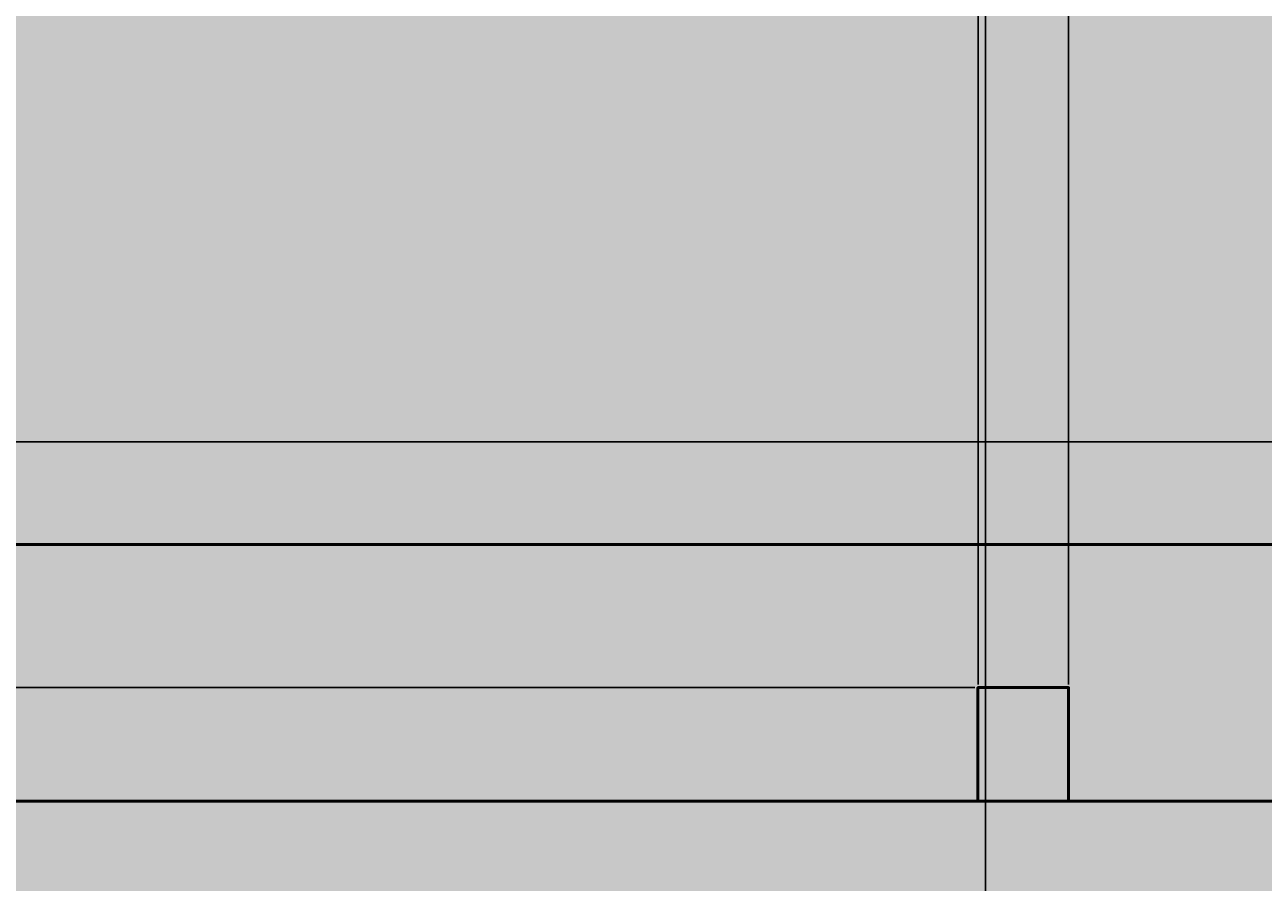
# Model space of a CAD drawing. Units: inches. Extents: x -12 to 334, y -10 to 186.
# Tile 53 of 77: x 198 to 222, y 94 to 111. Entities that reach past the tile are written whole.
import ezdxf

# ---------------------------------------------------------------- set-up
doc = ezdxf.new("R2010")
doc.units = ezdxf.units.IN
doc.header["$MEASUREMENT"] = 0
for name, color, linetype, lineweight in [('M-DIMS', 2, 'Continuous', 18), ('M-EQPM', 7, 'Continuous', 50), ('M-EQPM-PATT', 8, 'Continuous', 18)]:
    doc.layers.add(name, color=color, linetype=linetype, lineweight=lineweight)
doc.styles.get("Standard").update_dxf_attribs({"font": 'arial.ttf'})
doc.dimstyles.get("Standard").update_dxf_attribs({"dimtxt": 0.18, "dimasz": 0.18, "dimexe": 0.18, "dimexo": 0.0625, "dimgap": 0.09, "dimtad": 0, "dimtih": 1, "dimtoh": 1, "dimdec": 4, "dimzin": 0, "dimdsep": 46, "dimtxsty": 'Standard', "dimcen": 0.09, "dimadec": 0, "dimazin": 0, "dimtfac": 1, "dimtdec": 4, "dimtofl": 0, "dimtmove": 0, "dimatfit": 3, "dimfxl": 1, "dimtolj": 1, "dimtzin": 0, "dimarcsym": 0})

# ---------------------------------------------------------------- blocks, each defined once
blk = doc.blocks.new('*D17')
at = {"layer": 'Defpoints', "color": 0, "transparency": 16777216}
for p in [(106.177, 102.896), (105.892, 56.321), (295.976, 56.321)]:
    blk.add_point(p, dxfattribs=at)
at = {"layer": 'M-DIMS', "color": 0, "lineweight": -2, "transparency": 16777216}
for p, q in [((106.24, 102.896), (296.156, 102.896)), ((295.976, 102.716), (295.976, 79.79)), ((295.976, 56.501), (295.976, 79.426)), ((105.954, 56.321), (296.156, 56.321))]:
    blk.add_line(p, q, dxfattribs=at)
at = {"layer": 'M-DIMS', "color": 0, "transparency": 16777216}
for points in [[(295.946, 102.716), (296.006, 102.716), (295.976, 102.896)], [(295.946, 56.501), (296.006, 56.501), (295.976, 56.321)]]:
    blk.add_solid(points, dxfattribs=at)
at = {"layer": 'M-DIMS', "color": 0, "transparency": 16777216, "insert": (295.976, 79.608), "char_height": 0.18, "attachment_point": 5}
blk.add_mtext('\\A1;46.575', dxfattribs=at)
blk = doc.blocks.new('*D27')
at = {"layer": 'Defpoints', "color": 0, "transparency": 16777216}
for p in [(238.576, 169.385), (216.576, 32.854), (238.576, 32.854)]:
    blk.add_point(p, dxfattribs=at)
at = {"layer": 'M-DIMS', "color": 0, "lineweight": -2, "transparency": 16777216}
for p, q in [((216.576, 32.917), (216.576, 169.565)), ((238.576, 32.917), (238.576, 169.565)), ((216.756, 169.385), (227.357, 169.385)), ((238.396, 169.385), (227.796, 169.385))]:
    blk.add_line(p, q, dxfattribs=at)
at = {"layer": 'M-DIMS', "color": 0, "transparency": 16777216}
for points in [[(216.756, 169.415), (216.756, 169.355), (216.576, 169.385)], [(238.396, 169.415), (238.396, 169.355), (238.576, 169.385)]]:
    blk.add_solid(points, dxfattribs=at)
at = {"layer": 'M-DIMS', "color": 0, "transparency": 16777216, "insert": (227.576, 169.385), "char_height": 0.18, "attachment_point": 5}
blk.add_mtext('\\A1;22', dxfattribs=at)
blk = doc.blocks.new('*D34')
at = {"layer": 'Defpoints', "color": 0, "transparency": 16777216}
for p in [(218.192, 169.385), (216.428, 98.108), (218.192, 98.108)]:
    blk.add_point(p, dxfattribs=at)
at = {"layer": 'M-DIMS', "color": 0, "lineweight": -2, "transparency": 16777216}
for p, q in [((216.428, 98.171), (216.428, 169.565)), ((218.192, 98.171), (218.192, 169.565)), ((216.608, 169.385), (216.995, 169.385)), ((218.012, 169.385), (217.625, 169.385))]:
    blk.add_line(p, q, dxfattribs=at)
at = {"layer": 'M-DIMS', "color": 0, "transparency": 16777216}
for points in [[(216.608, 169.415), (216.608, 169.355), (216.428, 169.385)], [(218.012, 169.415), (218.012, 169.355), (218.192, 169.385)]]:
    blk.add_solid(points, dxfattribs=at)
at = {"layer": 'M-DIMS', "color": 0, "transparency": 16777216, "insert": (217.31, 169.385), "char_height": 0.18, "attachment_point": 5}
blk.add_mtext('\\A1;1.76', dxfattribs=at)
blk = doc.blocks.new('*D35')
at = {"layer": 'Defpoints', "color": 0, "transparency": 16777216}
for p in [(216.428, 98.108), (-11.174, 61.105), (216.428, 61.105)]:
    blk.add_point(p, dxfattribs=at)
at = {"layer": 'M-DIMS', "color": 0, "lineweight": -2, "transparency": 16777216}
for p, q in [((216.365, 98.108), (-11.354, 98.108)), ((-11.174, 97.928), (-11.174, 79.788)), ((-11.174, 61.285), (-11.174, 79.424)), ((216.365, 61.105), (-11.354, 61.105))]:
    blk.add_line(p, q, dxfattribs=at)
at = {"layer": 'M-DIMS', "color": 0, "transparency": 16777216}
for points in [[(-11.204, 97.928), (-11.144, 97.928), (-11.174, 98.108)], [(-11.204, 61.285), (-11.144, 61.285), (-11.174, 61.105)]]:
    blk.add_solid(points, dxfattribs=at)
at = {"layer": 'M-DIMS', "color": 0, "transparency": 16777216, "insert": (-11.174, 79.606), "char_height": 0.18, "attachment_point": 5}
blk.add_mtext('\\A1;37', dxfattribs=at)
blk = doc.blocks.new('*D40')
at = {"layer": 'Defpoints', "color": 0, "transparency": 16777216}
for p in [(278.229, 116.208), (187.394, 91.899)]:
    blk.add_point(p, dxfattribs=at)
at = {"layer": 'M-DIMS', "color": 0, "lineweight": -2, "transparency": 16777216}
for p, q in [((332.73, 130.793), (278.403, 116.254)), ((187.394, 91.809), (187.394, 91.989)), ((187.304, 91.899), (187.484, 91.899))]:
    blk.add_line(p, q, dxfattribs=at)
at = {"layer": 'M-DIMS', "color": 0, "transparency": 16777216}
blk.add_solid([(278.395, 116.283), (278.411, 116.225), (278.229, 116.208)], dxfattribs=at)
at = {"layer": 'M-DIMS', "color": 0, "transparency": 16777216, "insert": (333.21, 130.793), "char_height": 0.18, "attachment_point": 5}
blk.add_mtext('\\A1;R94.03', dxfattribs=at)

msp = doc.modelspace()

# ---------------------------------------------------------------- hatches: boundary and pattern name
at = {"layer": 'M-EQPM-PATT', "transparency": 33554556}
h = msp.add_hatch(color=256, dxfattribs=at)
h.set_gradient(color1=(248, 206, 179), color2=(248, 206, 179), tint=1)
h.paths.add_polyline_path([(179.7818, 136.8871), (126.9567, 136.8871), (106.1771, 100.8958), (171.5458, 100.8958)])
h.paths.add_polyline_path([(268.3808, 136.9435), (214.0166, 136.9435), (214.0166, 154.8345), (196.3421, 154.8345), (196.3421, 136.8871), (179.7818, 136.8871), (171.5458, 100.8958), (231.7758, 100.8958, -0.4142136), (251.9801, 80.6915), (279.7263, 80.6915, 0.1631825)])
at = {"layer": 'M-EQPM-PATT'}
h = msp.add_hatch(color=256, dxfattribs=at)
h.set_gradient(color1=(205, 32, 39), color2=(205, 32, 39), tint=1)
h.paths.add_polyline_path([(64.5, 80.754), (64.5, 89.8963), (226.6083, 89.8963, -1), (226.6083, 69.6117), (64.5, 69.6117), (64.5, 78.754), (4.4744, 78.754, 0.384914), (23.5807, 61.4872), (37.1002, 61.4872), (37.1002, 33.6752), (53.1002, 33.6752), (53.1002, 61.4872), (64.5, 61.4872), (64.5, 63.6117), (226.6083, 63.6117, 1), (226.6083, 95.8963), (64.5, 95.8963), (64.5, 99.8958), (53.1002, 99.8958), (53.1002, 127.7078), (37.1002, 127.7078), (37.1002, 99.8958), (23.5807, 99.8958, 0.4132606), (4.3766, 80.754)])
h.paths.add_polyline_path([(64.5, 91.8963), (64.5, 93.8963), (226.6083, 93.8963, -1), (226.6083, 65.6117), (64.5, 65.6117), (64.5, 67.6117), (226.6083, 67.6117, 1), (226.6083, 91.8963)], flags=16)
h = msp.add_hatch(color=256, dxfattribs=at)
h.set_gradient(color1=(99, 100, 102), color2=(99, 100, 102), tint=1)
h.paths.add_polyline_path([(72.9244, 95.8963), (75.9244, 95.8963), (75.9244, 109.0583), (72.9244, 109.0583)])
h.paths.add_polyline_path([(72.9244, 50.4497), (75.9244, 50.4497), (75.9244, 63.6117), (72.9244, 63.6117)])
h.paths.add_polyline_path([(75.9244, 91.8963), (75.9244, 93.8963), (72.9244, 93.8963), (72.9244, 91.8963)])
h.paths.add_polyline_path([(75.9244, 65.6117), (75.9244, 67.6117), (72.9244, 67.6117), (72.9244, 65.6117)])
h.paths.add_polyline_path([(129.093, 69.6117), (130.8573, 69.6117), (130.8573, 89.8963), (129.093, 89.8963)])
h.paths.add_polyline_path([(129.093, 98.1081), (129.093, 95.8963), (130.8573, 95.8963), (130.8573, 98.1081)])
h.paths.add_polyline_path([(130.8573, 61.1045), (130.8573, 63.6117), (129.093, 63.6117), (129.093, 61.1045)])
h.paths.add_polyline_path([(170.9079, 69.6117), (172.6722, 69.6117), (172.6722, 89.8963), (170.9079, 89.8963)])
h.paths.add_polyline_path([(172.6722, 95.8963), (172.6722, 98.1081), (170.9079, 98.1081), (170.9079, 95.8963)])
h.paths.add_polyline_path([(170.9079, 61.1045), (172.6722, 61.1045), (172.6722, 63.6117), (170.9079, 63.6117)])
h.paths.add_polyline_path([(218.1922, 63.6117), (216.4278, 63.6117), (216.4278, 61.1045), (218.1922, 61.1045)])
h.paths.add_polyline_path([(216.4278, 69.6117), (218.1922, 69.6117), (218.1922, 89.8963), (216.4278, 89.8963)])
h.paths.add_polyline_path([(216.4278, 95.8963), (218.1922, 95.8963), (218.1922, 98.1081), (216.4278, 98.1081)])
h = msp.add_hatch(color=256, dxfattribs=at)
h.set_gradient(color1=(94, 103, 175), color2=(94, 103, 175), tint=1)
h.paths.add_polyline_path([(129.093, 89.8963), (86.8879, 89.8963), (86.8879, 69.6117), (129.093, 69.6117)], flags=17)
h.paths.add_polyline_path([(170.9079, 89.8963), (130.8573, 89.8963), (130.8573, 69.6117), (170.9079, 69.6117)], flags=17)
h.paths.add_polyline_path([(216.4278, 89.8963), (172.6722, 89.8963), (172.6722, 69.6117), (216.4278, 69.6117)], flags=17)
h.paths.add_polyline_path([(245.9354, 82.6969), (247.9354, 82.6969), (247.9354, 46.8541), (268.3808, 46.8541, 0.0998398), (279.7263, 80.6915), (251.9801, 80.6915, 0.4142136), (231.7758, 100.8958), (84.7229, 100.8958), (84.7229, 109.0583), (83.7229, 109.0583), (83.7229, 95.8963), (129.093, 95.8963), (129.093, 98.1081), (130.8573, 98.1081), (130.8573, 95.8963), (170.9079, 95.8963), (170.9079, 98.1081), (172.6722, 98.1081), (172.6722, 95.8963), (216.4278, 95.8963), (216.4278, 98.1081), (218.1922, 98.1081), (218.1922, 95.8963), (226.6083, 95.8963, -1), (226.6083, 63.6117), (218.1922, 63.6117), (218.1922, 61.1045), (216.4278, 61.1045), (216.4278, 63.6117), (172.6722, 63.6117), (172.6722, 61.1045), (170.9079, 61.1045), (170.9079, 63.6117), (130.8573, 63.6117), (130.8573, 61.1045), (129.093, 61.1045), (129.093, 63.6117), (87.8879, 63.6117), (87.8879, 56.3205), (105.8919, 56.3205), (105.8919, 28.8541), (115.8919, 28.8541), (115.8919, 46.8541), (222.5761, 46.8541), (222.5761, 30.8541), (232.5761, 30.8541), (232.5761, 46.8541), (245.9354, 46.8541)])
h.paths.add_polyline_path([(86.8879, 89.8963), (75.9244, 89.8963), (75.9244, 69.6117), (86.8879, 69.6117)])
h.paths.add_polyline_path([(83.7229, 109.0583), (75.9244, 109.0583), (75.9244, 95.8963), (83.7229, 95.8963)])
h.paths.add_polyline_path([(226.6083, 89.8963), (218.1922, 89.8963), (218.1922, 69.6117), (226.6083, 69.6117, 1)], flags=17)
h = msp.add_hatch(color=256, dxfattribs=at)
h.set_gradient(color1=(0, 0, 255), color2=(0, 0, 255), tint=1)
h.paths.add_polyline_path([(84.7229, 100.8958), (84.7229, 109.0583), (83.7229, 109.0583), (83.7229, 95.8963), (129.093, 95.8963), (129.093, 98.1081), (130.8573, 98.1081), (130.8573, 95.8963), (170.9079, 95.8963), (170.9079, 98.1081), (172.6722, 98.1081), (172.6722, 95.8963), (216.4278, 95.8963), (216.4278, 98.1081), (218.1922, 98.1081), (218.1922, 95.8963), (226.6083, 95.8963, -1), (226.6083, 63.6117), (218.1922, 63.6117), (218.1922, 61.1045), (216.4278, 61.1045), (216.4278, 63.6117), (172.6722, 63.6117), (172.6722, 61.1045), (170.9079, 61.1045), (170.9079, 63.6117), (130.8573, 63.6117), (130.8573, 61.1045), (129.093, 61.1045), (129.093, 63.6117), (87.8879, 63.6117), (87.8879, 56.3205), (105.8919, 56.3205), (105.8919, 28.8541), (115.8919, 28.8541), (115.8919, 46.8541), (222.5761, 46.8541), (222.5761, 30.8541), (232.5761, 30.8541), (232.5761, 46.8541), (245.9354, 46.8541), (245.9354, 82.6969), (247.9354, 82.6969), (247.9354, 46.8541), (268.3808, 46.8541, 0.0998398), (279.7263, 80.6915), (251.9801, 80.6915, 0.4142136), (231.7758, 100.8958)])

# ---------------------------------------------------------------- linework, layer by layer
at = {"layer": 'M-EQPM'}
for points in [[(84.7229, 100.8958), (231.7758, 100.8958)], [(216.4278, 95.8963), (216.4278, 98.1081), (218.1922, 98.1081), (218.1922, 95.8963)]]:
    msp.add_lwpolyline(points, dxfattribs=at)
msp.add_lwpolyline([(64.5, 63.6117), (226.6083, 63.6117, 1), (226.6083, 95.8963), (64.5, 95.8963)], format="xyb", dxfattribs=at)

# ---------------------------------------------------------------- dimensions: what is measured, and where the dimension line sits
at = {"layer": 'M-DIMS'}
for base, p1, p2, override, picture, middle in [((218.1922, 169.3845), (216.4278, 98.1081), (218.1922, 98.1081), {"dimdec": 2, "dimlfac": 1, "dimrnd": 0, "dimzin": 0, "dimdsep": 46, "dimlunit": 2}, '*D34', (217.31, 169.3845)), ((238.5761, 169.3845), (216.5761, 32.8541), (238.5761, 32.8541), {"dimdec": 0, "dimlfac": 1, "dimrnd": 0, "dimzin": 0, "dimdsep": 46, "dimlunit": 2}, '*D27', (227.5761, 169.3845))]:
    dim = msp.add_linear_dim(base=base, p1=p1, p2=p2, dimstyle='Standard', override=override, dxfattribs=at)
    dim.commit()
    dim.dimension.update_dxf_attribs({"geometry": picture, "text_midpoint": middle})
dim = msp.add_radius_dim(center=(187.3936, 91.8988), mpoint=(278.2291, 116.2078), dimstyle='Standard', override={"dimdec": 2, "dimlfac": 1, "dimrnd": 0, "dimzin": 0, "dimdsep": 46, "dimlunit": 2}, dxfattribs=at)
dim.commit()
dim.dimension.update_dxf_attribs({"geometry": '*D40', "text_midpoint": (332.7304, 130.7932), "dimtype": 164})
for base, p1, p2, override, picture, middle in [((295.9756, 56.3205), (106.1771, 102.8958), (105.8919, 56.3205), {"dimdec": 3, "dimlfac": 1, "dimrnd": 0, "dimzin": 0, "dimdsep": 46, "dimlunit": 2}, '*D17', (295.9756, 79.6082)), ((-11.1736, 61.1045), (216.4278, 98.1081), (216.4278, 61.1045), {"dimdec": 0, "dimlfac": 1, "dimrnd": 0, "dimzin": 0, "dimdsep": 46, "dimlunit": 2}, '*D35', (-11.1735, 79.6063))]:
    dim = msp.add_linear_dim(base=base, p1=p1, p2=p2, angle=90, dimstyle='Standard', override=override, dxfattribs=at)
    dim.commit()
    dim.dimension.update_dxf_attribs({"geometry": picture, "text_midpoint": middle})

doc.saveas('drawing.dxf')
